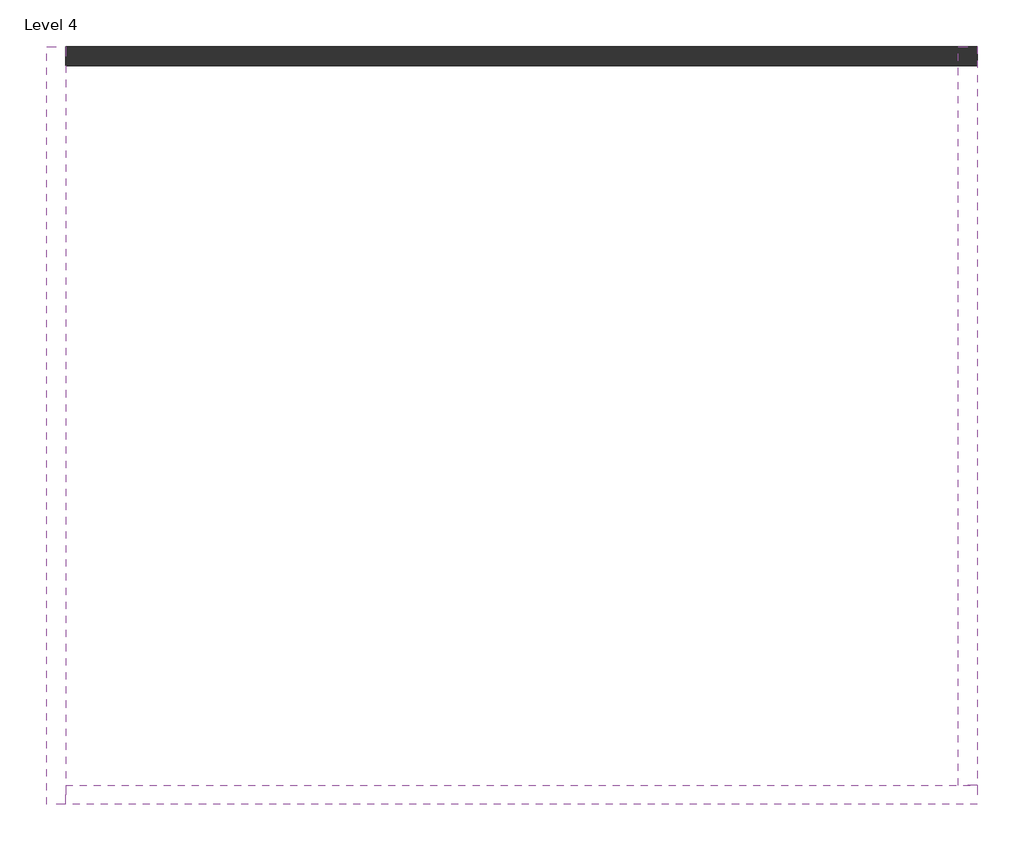
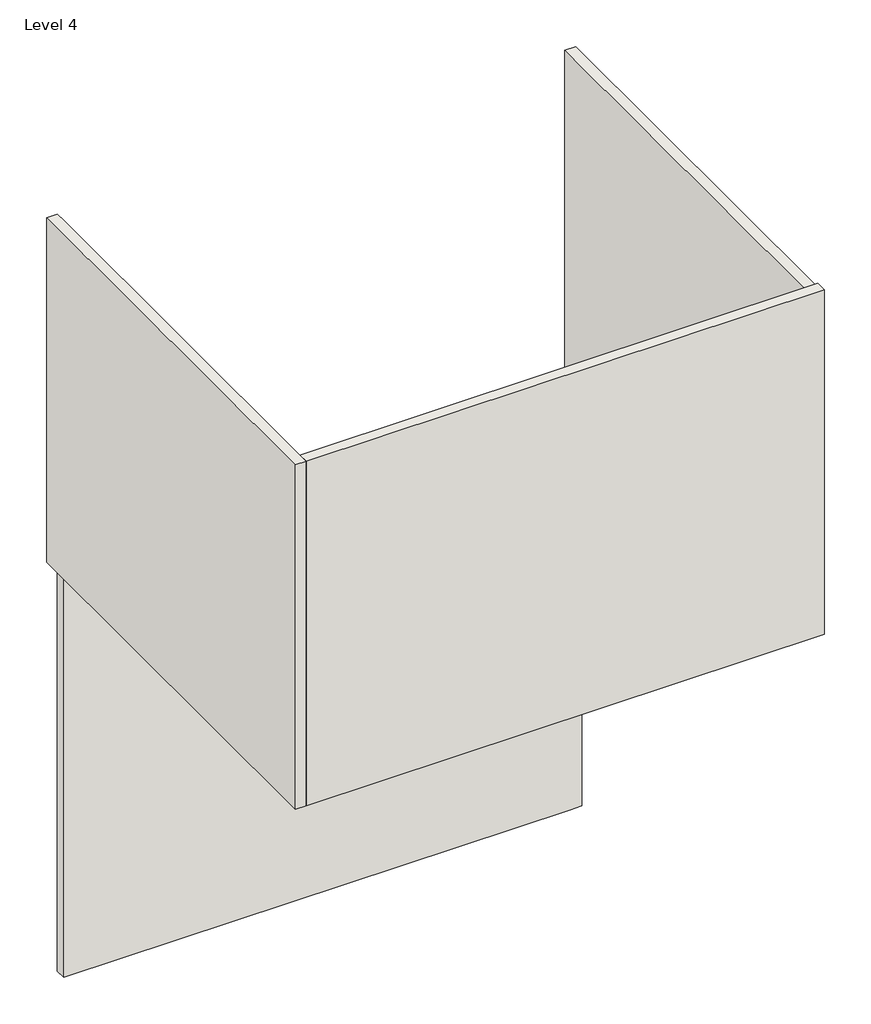
# One storey: 4 walls.
"""IFC4 building model written with IfcOpenShell, lengths in millimetres."""

from ifc_helpers import new_model, si_unit, frame, origin, place, context, project, spatial, polyline, outline, extrude, faceted_brep, element, save

model = new_model("IFC4")

# Units and contexts
model_context = context("Model", 3, world=origin())
ifc_project = project(units=[si_unit("LENGTHUNIT", "METRE", prefix="MILLI")], contexts=[model_context])

# Site, building, storey
site = spatial("IfcSite", under=ifc_project)
building = spatial("IfcBuilding", under=site)
storey = spatial("IfcBuildingStorey", under=building, Name="Level 4", Elevation=4000.0)

# Walls
placement = place(None, origin())
element("IfcWall", 1, ObjectType="Generic - 200mm", at=placement, inside=storey, context=model_context, shape_type="Brep", body=[
    faceted_brep([(-18302.079547, -9516.4007969, 18676.6324244), (-18302.079547, -9516.4007969, 13172.1483612), (-18302.079547, -9516.4007969, 12000.0), (-8802.079547, -9516.4007969, 12000.0), (-8802.079547, -9516.4007969, 18676.6324244), (-18302.079547, -9316.4007969, 12000.0), (-18302.079547, -9316.4007969, 18676.6324244), (-8802.079547, -9316.4007969, 18676.6324244), (-8802.079547, -9316.4007969, 18600.0), (-8802.079547, -9316.4007969, 12096.0), (-8802.079547, -9316.4007969, 12000.0)], [[[0, 1, 2, 3, 4]], [[5, 6, 7, 8, 9, 10]], [[3, 2, 5, 10]], [[0, 4, 7, 6]], [[4, 3, 10, 9, 8, 7]], [[0, 6, 5, 2, 1]]]),
])
element("IfcWall", 2, ObjectType="Generic - 200mm", at=placement, inside=storey, context=model_context, shape_type="Brep", body=[
    faceted_brep([(-18502.079547, -1616.4007969, 12000.0), (-18502.079547, -9516.4007969, 12000.0), (-18502.079547, -9516.4007969, 18676.6324244), (-18502.079547, -1616.4007969, 18676.6324244), (-18302.079547, -1616.4007969, 12000.0), (-18302.079547, -1616.4007969, 18676.6324244), (-18302.079547, -1816.4007969, 18676.6324244), (-18302.079547, -9316.4007969, 18676.6324244), (-18302.079547, -9516.4007969, 18676.6324244), (-18302.079547, -9516.4007969, 12000.0), (-18302.079547, -9316.4007969, 12000.0), (-18302.079547, -1816.4007969, 12000.0)], [[[0, 1, 2, 3]], [[4, 5, 6, 7, 8, 9, 10, 11]], [[1, 0, 4, 11, 10, 9]], [[3, 2, 8, 7, 6, 5]], [[1, 9, 8, 2]], [[0, 3, 5, 4]]]),
])
element("IfcWall", 3, ObjectType="Generic - 200mm", at=placement, inside=storey, context=model_context, shape_type="Brep", body=[
    faceted_brep([(-8802.079547, -1616.4007969, 4000.0), (-18302.079547, -1616.4007969, 4000.0), (-18302.079547, -1616.4007969, 12000.0), (-8802.079547, -1616.4007969, 12000.0), (-8802.079547, -1816.4007969, 4000.0), (-8802.079547, -1816.4007969, 12000.0), (-9002.079547, -1816.4007969, 12000.0), (-18302.079547, -1816.4007969, 12000.0), (-18302.079547, -1816.4007969, 4000.0), (-9002.079547, -1816.4007969, 4000.0)], [[[0, 1, 2, 3]], [[4, 5, 6, 7, 8, 9]], [[1, 0, 4, 9, 8]], [[3, 2, 7, 6, 5]], [[0, 3, 5, 4]], [[1, 8, 7, 2]]]),
])
element("IfcWall", 4, ObjectType="Generic - 200mm", at=placement, inside=storey, context=model_context, shape_type="SweptSolid", body=[
    extrude(outline(polyline([(-8802.079547, -1616.4007969), (-8802.079547, -9316.4007969), (-9002.079547, -9316.4007969), (-9002.079547, -1616.4007969), (-8802.079547, -1616.4007969)])), frame((0.0, 0.0, 12096.0), z_axis=(0.0, 0.0, 1.0), x_axis=(1.0, 0.0, 0.0)), (0.0, 0.0, 1.0), 6504.0),
])

save(model, "model.ifc")

# Revit data of these elements
# Type "Generic - 200mm"
#   Layers, outside or top first: 0' - 7.87402" no material (function 1)
# Elements 1, 2 (IfcWall, "Generic - 200mm")
#   built-in parameter 1001111 = 26' - 2.96063"
#   Top Offset = 0' - 0"
#   Base Offset = 26' - 2.96063"
#   Unconnected Height = 21' - 10.85954"
#   wall height = 21' - 10.85954"
#   Phase Created = New Construction
#   Base Constraint = Level 4
#   Materials on its faces: "Default Wall"
# Element 3 (IfcWall, "Generic - 200mm")
#   Top Offset = 0' - 0"
#   Base Offset = 0' - 0"
#   Unconnected Height = 26' - 2.96063"
#   wall height = 26' - 2.96063"
#   Phase Created = New Construction
#   Base Constraint = Level 4
#   Materials on its faces: "Default Wall"
# Element 4 (IfcWall, "Generic - 200mm")
#   built-in parameter 1001111 = 26' - 6.74016"
#   Top Offset = 0' - 0"
#   Base Offset = 26' - 6.74016"
#   Unconnected Height = 21' - 4.06299"
#   wall height = 21' - 4.06299"
#   Phase Created = New Construction
#   Base Constraint = Level 4
#   Materials on its faces: "Default Wall"
# Materials
#   "Default Wall": colour RGB 80 80 80, transparency 0
